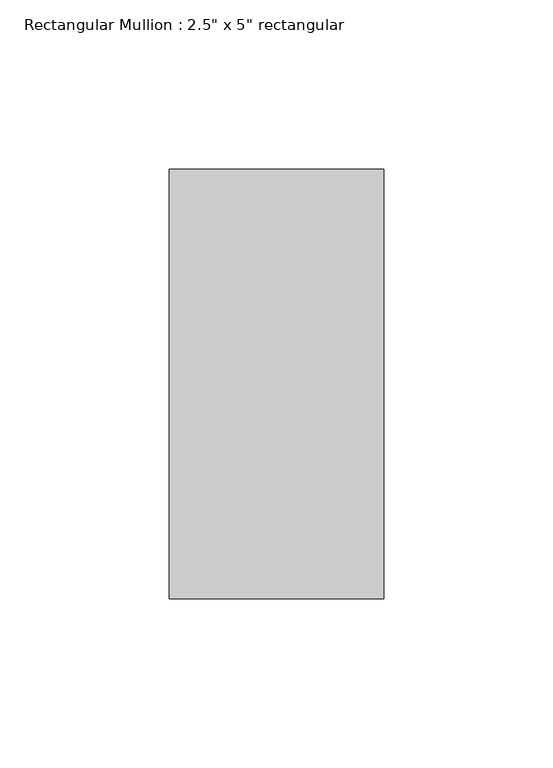
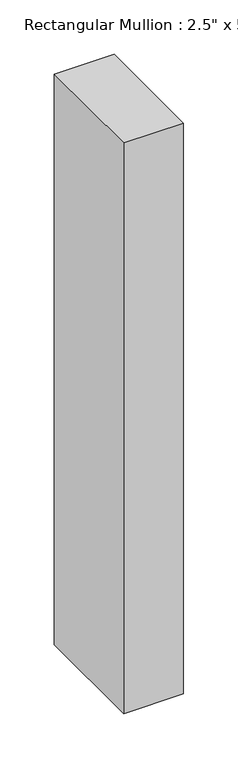
"""IFC4 building model written with IfcOpenShell, lengths in millimetres: member geometry."""

from ifc_helpers import new_model, si_unit, frame, origin, place, context, project, spatial, polyline, outline, extrude, source, transform, mapped, element, save


def member_e31b56d3(model_context):
    return source(origin(), model_context, "Body", "SweptSolid", [
        extrude(outline(polyline([(0.0, 63.5), (0.0, -63.5), (-63.5, -63.5), (-63.5, 63.5), (0.0, 63.5)])), frame((0.0, 0.0, -639.7075706), z_axis=(0.0, 0.0, 1.0), x_axis=(1.0, 0.0, 0.0)), (0.0, 0.0, 1.0), 639.7075706),
    ])


if __name__ == "__main__":
    model = new_model("IFC4")
    model_context = context("Model", 3, world=origin())
    ifc_project = project(units=[si_unit("LENGTHUNIT", "METRE", prefix="MILLI")], contexts=[model_context])
    site = spatial("IfcSite", under=ifc_project)
    building = spatial("IfcBuilding", under=site)
    placement = place(None, origin())
    member_shape = member_e31b56d3(model_context)
    element("IfcMember", 1, ObjectType="Rectangular Mullion : 2.5\" x 5\" rectangular", at=placement, inside=building, context=model_context, shape_type="MappedRepresentation", body=[
        mapped(member_shape, transform((0.0, 0.0, 0.0), x_axis=(1.0, 0.0, 0.0), y_axis=(0.0, 1.0, 0.0), z_axis=(0.0, 0.0, 1.0))),
    ])
    save(model, "model.ifc")

# Revit data of these elements
# Type "Rectangular Mullion : 2.5\" x 5\" rectangular"
#   built-in parameter 1007304 = 0.416667 (stored number, unit not read)
#   built-in parameter 1007301 = 0.104167 (stored number, unit not read)
#   built-in parameter 1007300 = 0.104167 (stored number, unit not read)
# Element 1 (IfcMember, "Rectangular Mullion : 2.5\" x 5\" rectangular")
#   Materials on its faces: "Aluminum"
# Materials
#   "Aluminum": class "Metal", colour RGB 247 247 247, transparency 0, Description = "Aluminum 6061", Cost = 0
